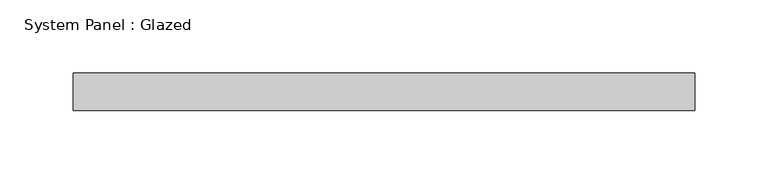
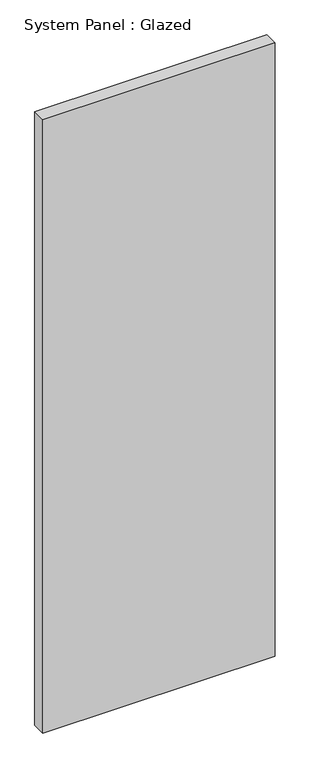
"""IFC4 building model written with IfcOpenShell, lengths in millimetres: plate geometry, System Panel : Glazed."""

from ifc_helpers import new_model, si_unit, origin, origin_with_axes, place, context, project, spatial, polyline, outline, extrude, source, transform, mapped, element, save


def system_panel_glazed_925bd09e(model_context):
    return source(origin(), model_context, "Body", "SweptSolid", [
        extrude(outline(polyline([(211.6666667, 19.05), (-211.6666667, 19.05), (-211.6666667, 44.45), (211.6666667, 44.45), (211.6666667, 19.05)])), origin_with_axes(), (0.0, 0.0, 1.0), 1181.1),
    ])


if __name__ == "__main__":
    model = new_model("IFC4")
    model_context = context("Model", 3, world=origin())
    ifc_project = project(units=[si_unit("LENGTHUNIT", "METRE", prefix="MILLI")], contexts=[model_context])
    site = spatial("IfcSite", under=ifc_project)
    building = spatial("IfcBuilding", under=site)
    placement = place(None, origin())
    system_panel_glazed_shape = system_panel_glazed_925bd09e(model_context)
    element("IfcPlate", 1, ObjectType="System Panel : Glazed", at=placement, inside=building, context=model_context, shape_type="MappedRepresentation", body=[
        mapped(system_panel_glazed_shape, transform((0.0, 0.0, 0.0), x_axis=(1.0, 0.0, 0.0), y_axis=(0.0, 1.0, 0.0), z_axis=(0.0, 0.0, 1.0))),
    ])
    save(model, "model.ifc")

# Revit data of these elements
# Type "System Panel : Glazed"
#   Construction Type Id = "GSP4R"
#   Analytic Construction = "1/8 in Pilkington single glazing"
#   Visual Light Transmittance = 0.9
#   Solar Heat Gain Coefficient = 0.86
#   Heat Transfer Coefficient (U) = 1.18115 BTU/(h·ft²·°F)
#   Define Thermal Properties by = 1
# Element 1 (IfcPlate, "System Panel : Glazed")
#   Materials on its faces: "Glass"
# Materials
#   "Glass": class "Glass", colour RGB 0 128 192, transparency 0.75, Description = "Soda Lime Glass", Cost = 0
